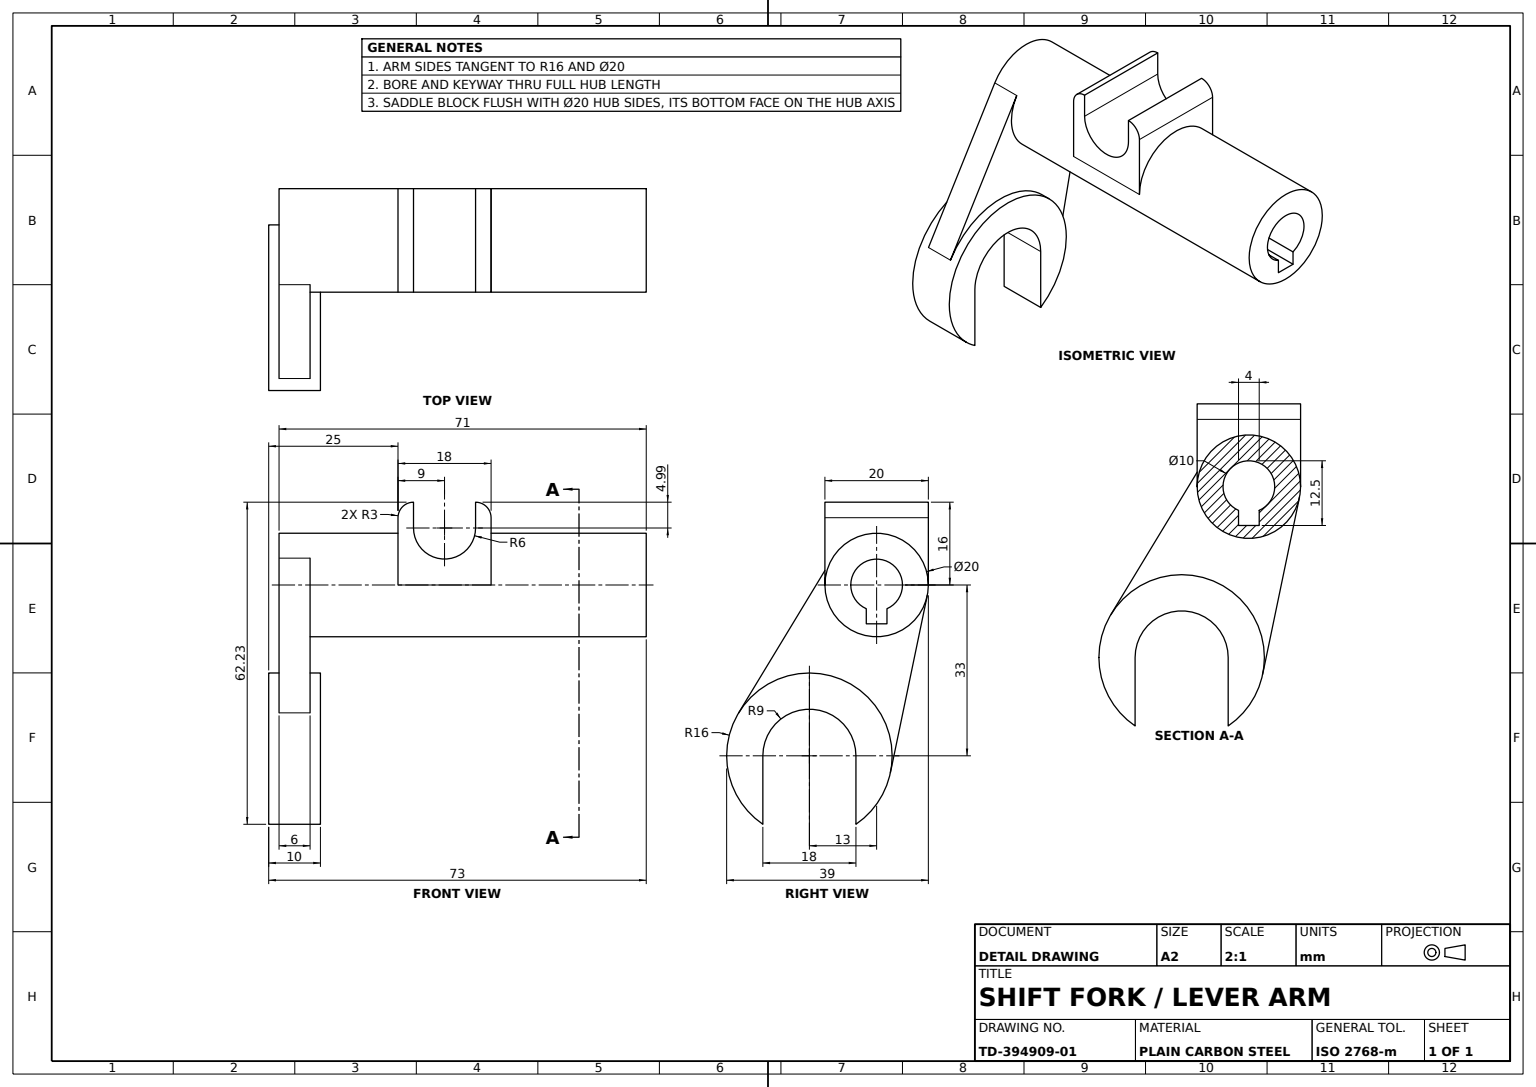
from build123d import *

# Parameters (mm, degrees)
HUB_PROFILE_20_R        = 10
SHAFT_HUB_20X71_DEPTH   = 71
KEYED_BORE_10_REACH     = 74.395
ROCKER_START            = -48
ROCKER_ARM_DEPTH        = 18
ARM_FILLET_R3_R         = 3
SADDLE_BLOCK_DEPTH      = 2
SADDLE_BLOCK_DEPTH_BACK = 8
CONNECTING_WEB_DEPTH    = 6
FORK_SLOT_DEPTH         = 90.549416149
FORK_SLOT_DEPTH_BACK    = 90.549416149


with BuildPart() as part:
    # Hub Profile Ø20 → Shaft Hub Ø20x71 (new body)
    with BuildSketch(Plane(origin=(0, 0, 0), x_dir=(0, 0, -1), z_dir=(1, 0, 0))):
        Circle(HUB_PROFILE_20_R)
    extrude(amount=SHAFT_HUB_20X71_DEPTH)

    # Keyed Bore Profile → Keyed Bore Ø10 (cut, up to next)
    with BuildSketch(Plane(origin=(71, 0, 0), x_dir=(0, 0, -1), z_dir=(1, 0, 0)), mode=Mode.PRIVATE) as keyed_bore_10_sk1:
        with BuildLine():
            Line((-2, -4.582575695), (-2, -7.5))
            Line((-2, -7.5), (2, -7.5))
            Line((2, -7.5), (2, -4.582575695))
            ThreePointArc((2, -4.582575695), (0, 5), (-2, -4.582575695))
        make_face()
    keyed_bore_10_tool1 = extrude(keyed_bore_10_sk1.sketch, amount=-KEYED_BORE_10_REACH, mode=Mode.PRIVATE) & part.part
    add(keyed_bore_10_tool1.solids().sort_by_distance((71, -0.731497, 0))[0], mode=Mode.SUBTRACT)

    # Rocker Arm Profile → Rocker Arm (add)
    with BuildSketch(Plane(origin=(71, 0, 0), x_dir=(0, 0, -1), z_dir=(1, 0, 0)).offset(ROCKER_START)):
        with BuildLine():
            Line((-10, 0), (-10, 16))
            Line((-10, 16), (10, 16))
            Line((10, 16), (10, 0))
            ThreePointArc((10, 0), (0, 10), (-10, 0))
        make_face()
    extrude(amount=ROCKER_ARM_DEPTH)

    # Arm Fillet R3
    arm_fillet_r3_edges = [part.edges().sort_by_distance(p)[0] for p in [
        (23, 16, 0),
        (41, 16, 0),
    ]]
    fillet(arm_fillet_r3_edges, radius=ARM_FILLET_R3_R)



with BuildPart() as body_2:
    # Saddle Block Profile → Saddle Block (new, two sides: drawn at the far end of the back side and taken through both)
    with BuildSketch(Plane.ZY.offset(-SADDLE_BLOCK_DEPTH_BACK)):
        with BuildLine():
            Line((22, -33), (22, -46.228756555))
            ThreePointArc((22, -46.228756555), (13, -17), (4, -46.228756555))
            Line((4, -46.228756555), (4, -33))
            ThreePointArc((4, -33), (13, -24), (22, -33))
        make_face()
    extrude(amount=SADDLE_BLOCK_DEPTH + SADDLE_BLOCK_DEPTH_BACK)


with BuildPart() as part_1:
    add(part.part)

    add(body_2.part)  # Connecting Web merges body 2
    # Connecting Web Profile → Connecting Web (add)
    with BuildSketch(Plane.ZY):
        with BuildLine():
            ThreePointArc((-2.664036214, -36.261590024), (7.135607706, -18.113465715), (26.679934465, -24.701843999))
            Line((26.679934465, -24.701843999), (8.549959041, 5.186347501))
            ThreePointArc((8.549959041, 5.186347501), (9.63066951, 2.692620433), (10, 0))
            ThreePointArc((10, 0), (1.024639854, -9.947367148), (-9.790022634, -2.038493765))
            Line((-9.790022634, -2.038493765), (-2.664036214, -36.261590024))
        make_face()
    extrude(amount=-CONNECTING_WEB_DEPTH)

    # Fork Slot Profile → Fork Slot (cut, two sides: drawn at the far end of the back side and taken through both)
    with BuildSketch(Plane.XY.offset(-FORK_SLOT_DEPTH_BACK)):
        with BuildLine():
            Line((26, 16), (26, 11.01))
            ThreePointArc((26, 11.01), (32, 5.01), (38, 11.01))
            Line((38, 11.01), (38, 16))
            Line((38, 16), (26, 16))
        make_face()
    extrude(amount=FORK_SLOT_DEPTH + FORK_SLOT_DEPTH_BACK, mode=Mode.SUBTRACT)


solid = part_1.part
